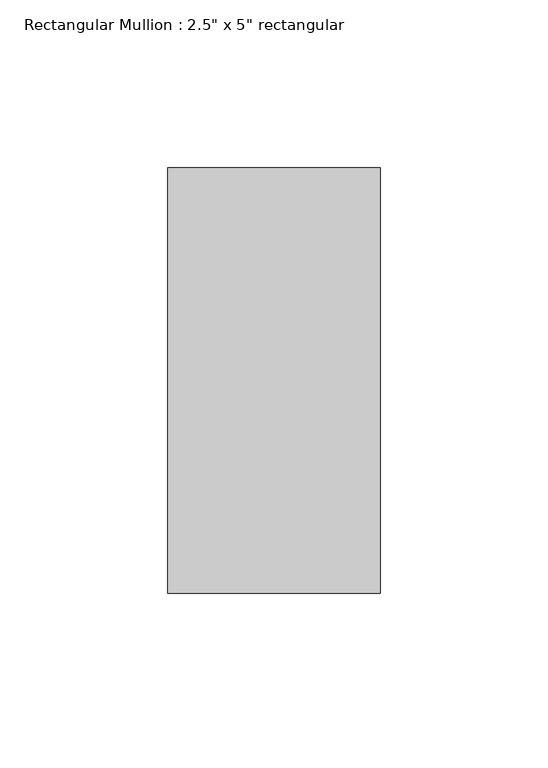
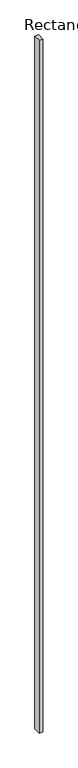
"""IFC4 building model written with IfcOpenShell, lengths in millimetres: member geometry."""

from ifc_helpers import new_model, si_unit, frame, origin, place, context, project, spatial, polyline, outline, extrude, source, transform, mapped, element, save


def member_dd9ec6c9(model_context):
    return source(origin(), model_context, "Body", "SweptSolid", [
        extrude(outline(polyline([(0.0, 63.5), (0.0, -63.5), (-63.5, -63.5), (-63.5, 63.5), (0.0, 63.5)])), frame((0.0, 0.0, -12758.7552746), z_axis=(0.0, 0.0, 1.0), x_axis=(1.0, 0.0, 0.0)), (0.0, 0.0, 1.0), 12758.7552746),
    ])


if __name__ == "__main__":
    model = new_model("IFC4")
    model_context = context("Model", 3, world=origin())
    ifc_project = project(units=[si_unit("LENGTHUNIT", "METRE", prefix="MILLI")], contexts=[model_context])
    site = spatial("IfcSite", under=ifc_project)
    building = spatial("IfcBuilding", under=site)
    placement = place(None, origin())
    member_shape = member_dd9ec6c9(model_context)
    element("IfcMember", 1, ObjectType="Rectangular Mullion : 2.5\" x 5\" rectangular", at=placement, inside=building, context=model_context, shape_type="MappedRepresentation", body=[
        mapped(member_shape, transform((0.0, 0.0, 0.0), x_axis=(1.0, 0.0, 0.0), y_axis=(0.0, 1.0, 0.0), z_axis=(0.0, 0.0, 1.0))),
    ])
    save(model, "model.ifc")

# Revit data of these elements
# Type "Rectangular Mullion : 2.5\" x 5\" rectangular"
#   built-in parameter 1007304 = 0.416667 (stored number, unit not read)
#   built-in parameter 1007301 = 0.104167 (stored number, unit not read)
#   built-in parameter 1007300 = 0.104167 (stored number, unit not read)
# Element 1 (IfcMember, "Rectangular Mullion : 2.5\" x 5\" rectangular")
#   Materials on its faces: "Aluminum"
# Materials
#   "Aluminum": class "Metal", colour RGB 247 247 247, transparency 0, Description = "Aluminum 6061", Cost = 0
